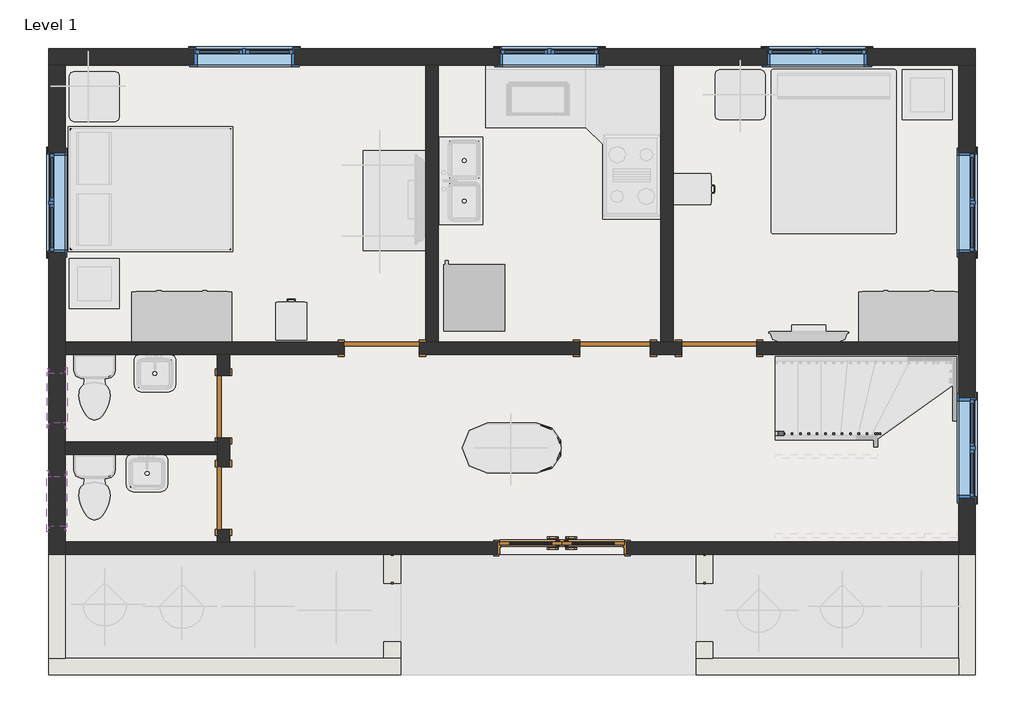
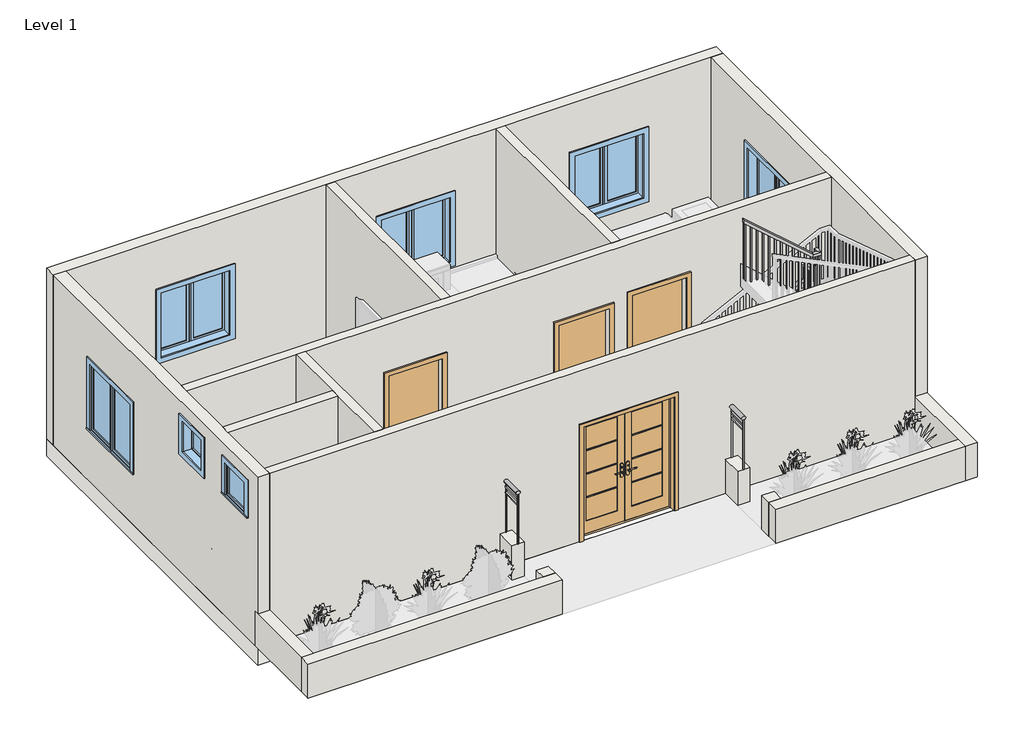
# One storey, part 1 of 2: 17 walls, 8 windows, 6 doors, 3 railings, 1 slab.
# Revit data of these elements (continued)
# Element 33 (IfcWindow, "Casement Dbl with Trim : 48\" x 48\"")
#   Mark = "6"
#   Phase Created = New Construction
#   Materials on its faces: "Sash", "Trim", "Glass"
# Element 34 (IfcWindow, "Transom with Trim : 24\" x 24\"")
#   Mark = "7"
#   Phase Created = New Construction
#   Materials on its faces: "Sash", "Trim", "Glass"
# Element 35 (IfcWindow, "Transom with Trim : 24\" x 24\"")
#   Mark = "8"
#   Phase Created = New Construction
#   Materials on its faces: "Sash", "Trim", "Glass"
# Materials
#   "Cherry": class "Wood", colour RGB 226 177 128, transparency 0, Description = "Prunus Serotina", Cost = 0
#   "Glass": class "Glass", colour RGB 0 128 192, transparency 0.75, Description = "Soda Lime Glass", Cost = 0
#   "Aluminum": class "Metal", colour RGB 247 247 247, transparency 0, Description = "Aluminum 6061", Cost = 0
#   "Door - Panel": class "Wood", colour RGB 210 159 95, transparency 0
#   "Door - Frame": colour RGB 118 70 51, transparency 0
#   "Birch": class "Wood", colour RGB 224 178 126, transparency 0, Description = "Betula Alleghaniensis", Cost = 0
#   "Brick, Common": class "Masonry", colour RGB 170 98 104, transparency 0, Description = "Common brick", Cost = 0
#   "Sash": class "Wood", colour RGB 224 178 126, transparency 0
#   "Trim": class "Wood", colour RGB 224 178 126, transparency 0
#   "Default Floor": colour RGB 128 128 128, transparency 0
# Room at (-12043.468, 12435.992) mm, phase "New Construction", upper level "Level 1", upper offset 10' - 0", lower offset 0' - 0"
#   Number = "1"
#   Name = "BEDROOM"
# Room at (-8131.24, 12435.992) mm, phase "New Construction", upper level "Level 1", upper offset 10' - 0", lower offset 0' - 0"
#   Number = "2"
#   Name = "BEDROOM"
# Room at (-4587.108, 12288.469) mm, phase "New Construction", upper level "Level 1", upper offset 10' - 0", lower offset 0' - 0"
#   Number = "3"
#   Name = "BEDROOM"
# Room at (-13236.413, 9824.071) mm, phase "New Construction", upper level "Level 1", upper offset 10' - 0", lower offset 0' - 0"
#   Number = "4"
#   Name = "BATH"
# Room at (-13310.931, 8635.704) mm, phase "New Construction", upper level "Level 1", upper offset 10' - 0", lower offset 0' - 0"
#   Number = "5"
#   Name = "BATH"
# Room at (-7548.719, 9201.62) mm, phase "New Construction", upper level "Level 1", upper offset 10' - 0", lower offset 0' - 0"
#   Number = "6"
#   Name = "LOBBY"
